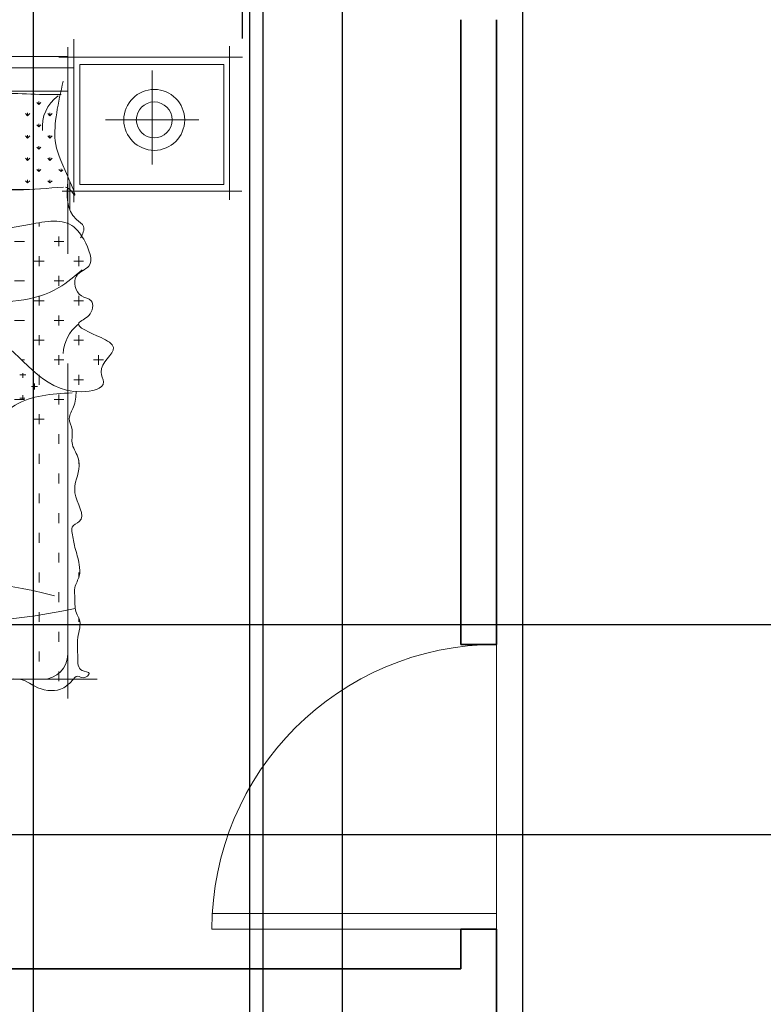
# Model space of a CAD drawing. Units: inches. Extents: x -438 to 102, y -60 to 1091.
# Tile 13 of 20: x -243 to -149, y 898 to 1022. Entities that reach past the tile are written whole.
import ezdxf

# ---------------------------------------------------------------- set-up
doc = ezdxf.new("R2010")
doc.units = ezdxf.units.IN
doc.header["$MEASUREMENT"] = 0
for name, color, linetype, lineweight, true_color in [('A-ANNO-DIMS', 217, 'Continuous', 18, 0x93278f), ('A-DOOR', 30, 'Continuous', 18, 0xf26722), ('A-WALL', 2, 'Continuous', 35, 0xf1eb1f)]:
    doc.layers.add(name, color=color, linetype=linetype, lineweight=lineweight, true_color=true_color)
doc.layers.add('Furniture', color=7, linetype='Continuous', lineweight=15)
doc.styles.get("Standard").update_dxf_attribs({"font": 'arial.ttf'})
doc.dimstyles.get("Standard").update_dxf_attribs({"dimtxt": 8, "dimasz": 0.18, "dimexe": 0.18, "dimexo": 0.0625, "dimgap": 0.09, "dimtad": 0, "dimtih": 1, "dimtoh": 1, "dimdec": 4, "dimzin": 0, "dimdsep": 46, "dimlunit": 3, "dimtxsty": 'Standard', "dimcen": 0.09, "dimadec": 0, "dimazin": 0, "dimtfac": 1, "dimtdec": 4, "dimtofl": 0, "dimtmove": 0, "dimatfit": 3, "dimfxl": 1, "dimtolj": 1, "dimtzin": 0, "dimarcsym": 0})

# ---------------------------------------------------------------- blocks, each defined once
blk = doc.blocks.new('BED-DOUBLE-WITH-NIGHTSTANDS')
for p, q in [((30.68, 0), (30.68, -20.6)), ((29.9, -1.01), (29.9, -27.13)), ((50.37, -20.33), (50.37, -0.9)), ((-30.74, -2.19), (29.9, -2.19)), ((51.99, -2.28), (28.76, -2.28)), ((30.68, -3.64), (-30.92, -3.64)), ((49.65, -3.21), (31.43, -3.21)), ((31.43, -3.21), (31.43, -18.39)), ((49.65, -18.39), (49.65, -3.21)), ((40.58, -3.96), (40.58, -15.85)), ((29.9, -6.59), (7.41, -6.59)), ((26.23, -8.26), (25.97, -8)), ((26.23, -8.27), (26.23, -7.89)), ((26.23, -8.26), (26.5, -8)), ((24.82, -9.68), (24.55, -9.41)), ((24.82, -9.68), (24.82, -9.3)), ((24.82, -9.68), (25.08, -9.41)), ((27.65, -9.68), (27.38, -9.41)), ((27.65, -9.68), (27.65, -9.3)), ((27.65, -9.68), (27.91, -9.41)), ((26.23, -11.09), (25.97, -10.83)), ((26.23, -11.09), (26.23, -10.72)), ((26.23, -11.09), (26.5, -10.83)), ((46.48, -10.21), (34.68, -10.21)), ((24.82, -12.51), (24.55, -12.24)), ((24.82, -12.51), (24.82, -12.13)), ((24.82, -12.51), (25.08, -12.24)), ((27.65, -12.51), (27.38, -12.24)), ((27.65, -12.51), (27.65, -12.13)), ((27.65, -12.51), (27.91, -12.24)), ((26.23, -13.92), (25.97, -13.66)), ((26.23, -13.92), (26.23, -13.55)), ((26.23, -13.92), (26.5, -13.66)), ((24.82, -15.34), (24.55, -15.07)), ((24.82, -15.34), (24.82, -14.96)), ((24.82, -15.34), (25.08, -15.07)), ((27.65, -15.34), (27.38, -15.07)), ((27.65, -15.34), (27.65, -14.96)), ((27.65, -15.34), (27.91, -15.07)), ((26.23, -16.75), (25.97, -16.48)), ((26.23, -16.75), (26.23, -16.38)), ((26.23, -16.75), (26.5, -16.48)), ((29.06, -16.75), (28.79, -16.48)), ((29.06, -16.75), (29.06, -16.38)), ((29.06, -16.75), (29.27, -16.54)), ((24.82, -18.16), (24.55, -17.9)), ((24.82, -18.16), (24.82, -17.79)), ((24.82, -18.16), (25.08, -17.9)), ((27.65, -18.16), (27.38, -17.9)), ((27.65, -18.16), (27.65, -17.79)), ((27.65, -18.16), (27.91, -17.9)), ((30.17, -21.62), (30.17, -17.94)), ((31.43, -18.39), (49.65, -18.39)), ((29.21, -19.21), (51.9, -19.21)), ((26.28, -23.69), (26.28, -23.21)), ((24.41, -25.57), (23.16, -25.57)), ((29.41, -25.57), (28.16, -25.57)), ((28.78, -26.19), (28.78, -24.94)), ((26.91, -28.07), (25.66, -28.07)), ((26.28, -28.69), (26.28, -27.44)), ((31.91, -28.07), (30.66, -28.07)), ((31.28, -28.69), (31.28, -27.44)), ((24.41, -30.57), (23.16, -30.57)), ((29.41, -30.57), (28.16, -30.57)), ((28.78, -31.19), (28.78, -29.94)), ((26.91, -33.07), (25.66, -33.07)), ((26.28, -33.69), (26.28, -32.44)), ((31.91, -33.07), (30.66, -33.07)), ((31.28, -33.69), (31.28, -32.44)), ((24.41, -35.57), (23.16, -35.57)), ((29.41, -35.57), (28.16, -35.57)), ((28.78, -36.19), (28.78, -34.94)), ((26.91, -38.07), (25.66, -38.07)), ((26.28, -38.69), (26.28, -37.44)), ((31.91, -38.07), (30.66, -38.07)), ((31.28, -38.69), (31.28, -37.44)), ((24.41, -40.57), (24.09, -40.57)), ((29.41, -40.57), (28.16, -40.57)), ((28.78, -41.19), (28.78, -39.94)), ((29.9, -41), (29.9, -83.36)), ((34.41, -40.57), (33.16, -40.57)), ((33.78, -41.19), (33.78, -39.94)), ((24.22, -42.82), (24.22, -42.22)), ((24.59, -42.45), (23.85, -42.45)), ((25.7, -44.29), (25.7, -43.56)), ((26.28, -43.69), (26.28, -42.44)), ((31.91, -43.07), (30.66, -43.07)), ((31.28, -43.69), (31.28, -42.44)), ((26.07, -43.92), (25.33, -43.92)), ((24.41, -45.57), (23.16, -45.57)), ((24.47, -45.4), (23.85, -45.4)), ((24.22, -45.56), (24.22, -45.03)), ((29.41, -45.57), (28.16, -45.57)), ((28.78, -46.19), (28.78, -44.94)), ((26.91, -48.07), (25.66, -48.07)), ((26.28, -48.69), (26.28, -47.44)), ((28.78, -51.19), (28.78, -49.94)), ((26.28, -53.69), (26.28, -52.44)), ((31.28, -53.69), (31.28, -53.25)), ((28.78, -56.19), (28.78, -54.94)), ((26.28, -58.69), (26.28, -57.44)), ((28.78, -61.19), (28.78, -59.94)), ((26.28, -63.69), (26.28, -62.44)), ((28.78, -66.19), (28.78, -64.94)), ((26.28, -68.69), (26.28, -67.44)), ((31.28, -68.1), (31.28, -67.44)), ((28.78, -71.19), (28.78, -69.94)), ((26.28, -73.69), (26.28, -72.44)), ((31.28, -73.69), (31.28, -73.16)), ((28.78, -76.19), (28.78, -74.94)), ((26.28, -78.69), (26.28, -77.44)), ((28.78, -81.19), (28.78, -79.94)), ((33.6, -80.93), (-28.29, -80.93))]:
    blk.add_line(p, q)
for radius in [3.85, 2.27]:
    blk.add_circle((40.84, -10.21), radius)
for centre, radius, start, end in [((31.35, -11.01), 4.66, 124.7345, 186.5526), ((24.21, 1.34), 20.36, 248.1857, 275.9106), ((34.27, -39.94), 4.94, 128.8354, 178.0038), ((14.99, -0.75), 72.97, 239.8126, 282.5472), ((9.5, -143.88), 75.85, 75.7143, 109.4459), ((26.75, -77.78), 3.15, 270, 0)]:
    blk.add_arc(centre, radius, start, end)
for points, knots in [([(29.35, -18.7), (25.48, -19.02), (19.22, -19.53), (10.28, -16.58), (3.99, -20.47), (0.06, -17.44), (0.95, -13.79), (1.87, -10.79), (0.46, -7.43), (6.72, -5.67), (11.66, -7.91), (18.15, -7.12), (22.47, -6.73), (26.14, -7.04), (28.33, -7.01), (29.06, -7.01)], [0, 0, 0, 0, 11.502554, 18.635017, 27.654655, 28.800011, 32.595859, 36.914018, 38.927328, 41.544104, 52.009639, 56.262652, 60.661637, 65.075538, 67.252844, 67.252844, 67.252844, 67.252844]), ([(29.32, -5.32), (28.7, -8.05), (27.69, -12.51), (29.2, -15.74), (31.39, -20.84), (30.11, -18.79), (29.6, -18.7)], [0, 0, 0, 0, 7.603099, 12.404488, 14.892294, 16.432626, 16.432626, 16.432626, 16.432626]), ([(29.9, -17.94), (29.78, -19.78), (29.64, -22.09), (32.27, -23.65), (31.79, -24.62), (31.53, -25.14)], [0, 0, 0, 0, 4.973031, 6.254082, 7.747585, 7.747585, 7.747585, 7.747585]), ([(31.93, -25.29), (32.57, -26.62), (33.59, -28.72), (30.29, -29.71), (31.01, -32.64), (33.35, -32.83), (32.92, -35.12), (30.08, -36.11), (33.79, -37.48), (36.78, -39.18), (33.39, -41.32), (35.07, -44.06), (26.87, -46.02), (20.99, -32.35), (2.1, -54.12), (-16.08, -50.43), (-31.16, -41.37), (-34.82, -50.79), (-35.75, -45.56), (-33.27, -44.57), (-36.07, -39.92), (-29.61, -39.91), (-31.05, -37.18), (-31.79, -35.41), (-31.67, -30.43), (-16.86, -30.76), (-35.73, -24.41), (-25.68, -23.88), (-16.82, -24.97), (2.34, -26.69), (17.46, -24.9), (30.09, -22.48), (31.54, -24.71), (31.93, -25.29)], [0, 0, 0, 0, 3.481099, 5.475811, 8.043407, 9.436812, 11.330727, 12.888379, 16.258255, 18.252967, 21.734596, 23.018392, 26.087149, 38.445812, 54.5649, 86.600283, 92.594507, 98.286547, 100.905288, 101.70342, 105.471876, 109.954916, 110.954151, 113.598333, 116.114301, 124.231953, 133.25029, 137.509046, 143.991555, 164.906349, 189.961005, 195.579007, 197.573325, 197.573325, 197.573325, 197.573325]), ([(31.74, -29.16), (30.78, -29.98), (26.99, -33.22), (21.81, -33.32), (17.94, -33.4)], [0, 0, 0, 0, 3.737027, 14.742384, 14.742384, 14.742384, 14.742384]), ([(30.47, -44.73), (27.88, -44.87), (22.83, -45.15), (16.72, -54.5), (5.64, -51.25), (-8.89, -48.66), (-19.85, -50.38), (-33.1, -52.54), (-34.5, -49.21), (-35, -48.01)], [0, 0, 0, 0, 7.385187, 14.402621, 29.694422, 35.583277, 59.348121, 65.733553, 69.320983, 69.320983, 69.320983, 69.320983]), ([(30.96, -44.51), (30.93, -45.19), (30.86, -46.38), (29.77, -47.93), (30.68, -49.44), (30.18, -51.19), (31.18, -52.55), (31.56, -54.75), (29.86, -57.22), (32.61, -60.74), (30.28, -61.5), (30.52, -62.88), (30.79, -64.38), (31.38, -66.15), (31.51, -67.95), (30.62, -69.27), (30.89, -70.9), (30.72, -72.32), (31.74, -73.74), (30.93, -75.81), (31.25, -77.78), (31.09, -79.97), (33.09, -80.01), (31.89, -81), (31.1, -80.32), (30.21, -81.43), (28.73, -82.66), (26.29, -82.31), (24.17, -80.73), (21.7, -80.78), (19.49, -82.4), (17.06, -81.88), (13.17, -82.17), (8.82, -81.36), (4.07, -80.77), (0.46, -83.09), (-2.79, -81.85), (-5.87, -81.65), (-14.3, -79.69), (-20.14, -80.18), (-31.55, -83.45), (-29.78, -79.6), (-32.81, -83.8), (-29.07, -82.96), (-24.85, -82.73), (-30.36, -81.5), (-32.31, -79.09), (-32.11, -72.2), (-27.72, -79.52), (-31.69, -72.6), (-28.72, -70.51), (-27.65, -65.93), (-35.2, -65.77), (-26.02, -64.12), (-35.79, -62.68), (-27.32, -61.35), (-31.95, -58.4), (-27.39, -55.21), (-31.95, -53.76), (-28.5, -51.75), (-29.55, -48.81), (-29.07, -42.18), (-29.13, -46.29), (-29.16, -48.01)], [0, 0, 0, 0, 2.033881, 3.581387, 5.07489, 6.704853, 8.655612, 9.757262, 13.24098, 16.903694, 18.063816, 18.788243, 20.635227, 22.875483, 24.324336, 25.871843, 27.320698, 29.140811, 29.950855, 32.312207, 34.847704, 36.565952, 37.541804, 38.447727, 39.194923, 40.100844, 41.912688, 45.194843, 46.251388, 49.875946, 51.496686, 54.215105, 56.7523, 63.316606, 67.484853, 70.581422, 75.324573, 76.965649, 79.915763, 100.671038, 102.483321, 104.317501, 106.523635, 109.038061, 111.571263, 115.809372, 117.667229, 122.411431, 125.445794, 129.976907, 132.758854, 136.424739, 139.918708, 143.481583, 147.135325, 151.002466, 153.252794, 157.23352, 159.244583, 161.905351, 164.097269, 169.015093, 172.531686, 172.531686, 172.531686, 172.531686])]:
    blk.add_open_spline(points, degree=3, knots=knots)
blk = doc.blocks.new('DOOR-SWING-36')
for p, q in [((-36, 0), (0, 0)), ((-2, 0), (-2, -36)), ((0, 0), (0, -36))]:
    blk.add_line(p, q)
blk.add_arc((0, 0), 36, 180, 270)
blk = doc.blocks.new('*D12')
at = {"layer": 'A-ANNO-DIMS', "color": 0, "lineweight": -2, "transparency": 16777216}
for p, q in [((-319.27, 1020.11), (-319.27, 1035.82)), ((-319.09, 1035.64), (-304.62, 1035.64)), ((-215.48, 1035.64), (-229.95, 1035.64)), ((-215.3, 1020.11), (-215.3, 1035.82))]:
    blk.add_line(p, q, dxfattribs=at)
at = {"layer": 'A-ANNO-DIMS', "color": 0, "transparency": 16777216}
for points in [[(-319.09, 1035.67), (-319.09, 1035.61), (-319.27, 1035.64)], [(-215.48, 1035.67), (-215.48, 1035.61), (-215.3, 1035.64)]]:
    blk.add_solid(points, dxfattribs=at)
at = {"layer": 'Defpoints', "color": 0, "transparency": 16777216}
for p in [(-215.3, 1035.64), (-319.27, 1020.04), (-215.3, 1020.04)]:
    blk.add_point(p, dxfattribs=at)
at = {"layer": 'A-ANNO-DIMS', "color": 0, "transparency": 16777216, "insert": (-267.28, 1035.64), "char_height": 8, "attachment_point": 5}
blk.add_mtext('\\A1;BED 8\'-8" TYP.', dxfattribs=at)
blk = doc.blocks.new('*D37')
at = {"layer": 'A-ANNO-DIMS', "color": 0, "lineweight": -2, "transparency": 16777216}
for p, q in [((-179.8, 234.94), (-179.8, 1079.58)), ((-134.08, 234.94), (-134.08, 1079.58)), ((-179.62, 1079.4), (-176.98, 1079.4)), ((-134.26, 1079.4), (-136.9, 1079.4))]:
    blk.add_line(p, q, dxfattribs=at)
at = {"layer": 'A-ANNO-DIMS', "color": 0, "transparency": 16777216}
for points in [[(-179.62, 1079.43), (-179.62, 1079.37), (-179.8, 1079.4)], [(-134.26, 1079.43), (-134.26, 1079.37), (-134.08, 1079.4)]]:
    blk.add_solid(points, dxfattribs=at)
at = {"layer": 'Defpoints', "color": 0, "transparency": 16777216}
for p in [(-134.08, 1079.4), (-179.8, 234.88), (-134.08, 234.88)]:
    blk.add_point(p, dxfattribs=at)
at = {"layer": 'A-ANNO-DIMS', "color": 0, "transparency": 16777216, "insert": (-156.94, 1079.4), "char_height": 8, "attachment_point": 5}
blk.add_mtext('\\A1;3\'-9 1/2"', dxfattribs=at)
blk = doc.blocks.new('*D44')
at = {"layer": 'A-ANNO-DIMS', "color": 0, "lineweight": -2, "transparency": 16777216}
for p, q in [((-64.71, 946), (-414.94, 946)), ((-414.76, 945.82), (-414.76, 936.94)), ((-414.76, 919.6), (-414.76, 928.48)), ((-64.71, 919.42), (-414.94, 919.42))]:
    blk.add_line(p, q, dxfattribs=at)
at = {"layer": 'A-ANNO-DIMS', "color": 0, "transparency": 16777216}
for points in [[(-414.79, 945.82), (-414.73, 945.82), (-414.76, 946)], [(-414.79, 919.6), (-414.73, 919.6), (-414.76, 919.42)]]:
    blk.add_solid(points, dxfattribs=at)
at = {"layer": 'Defpoints', "color": 0, "transparency": 16777216}
for p in [(-64.65, 946), (-414.76, 919.42), (-64.65, 919.42)]:
    blk.add_point(p, dxfattribs=at)
at = {"layer": 'A-ANNO-DIMS', "color": 0, "transparency": 16777216, "insert": (-414.76, 932.71), "char_height": 8, "attachment_point": 5}
blk.add_mtext('\\A1;2\'-2 1/2"', dxfattribs=at)
blk = doc.blocks.new('*D53')
at = {"layer": 'A-ANNO-DIMS', "color": 0, "lineweight": -2, "transparency": 16777216}
for p, q in [((-241.7, 824.44), (-241.7, 1079.58)), ((-214.37, 824.44), (-214.37, 1079.58)), ((-241.52, 1079.4), (-214.55, 1079.4)), ((-214.37, 1079.4), (-214.19, 1079.4))]:
    blk.add_line(p, q, dxfattribs=at)
at = {"layer": 'A-ANNO-DIMS', "color": 0, "transparency": 16777216}
for points in [[(-241.52, 1079.43), (-241.52, 1079.37), (-241.7, 1079.4)], [(-214.55, 1079.43), (-214.55, 1079.37), (-214.37, 1079.4)]]:
    blk.add_solid(points, dxfattribs=at)
at = {"layer": 'Defpoints', "color": 0, "transparency": 16777216}
for p in [(-214.37, 1079.4), (-241.7, 824.38), (-214.37, 824.38)]:
    blk.add_point(p, dxfattribs=at)
at = {"layer": 'A-ANNO-DIMS', "color": 0, "transparency": 16777216, "insert": (-194.08, 1079.4), "char_height": 8, "attachment_point": 5}
blk.add_mtext('\\A1;2\'-3 1/2"', dxfattribs=at)
blk = doc.blocks.new('*D61')
at = {"layer": 'A-ANNO-DIMS', "color": 0, "lineweight": -2, "transparency": 16777216}
for p, q in [((-212.65, 534.56), (-212.65, 1079.58)), ((-202.65, 534.56), (-202.65, 1079.58)), ((-212.65, 1079.4), (-212.83, 1079.4)), ((-202.83, 1079.4), (-212.47, 1079.4))]:
    blk.add_line(p, q, dxfattribs=at)
at = {"layer": 'A-ANNO-DIMS', "color": 0, "transparency": 16777216}
for points in [[(-212.47, 1079.43), (-212.47, 1079.37), (-212.65, 1079.4)], [(-202.83, 1079.43), (-202.83, 1079.37), (-202.65, 1079.4)]]:
    blk.add_solid(points, dxfattribs=at)
at = {"layer": 'Defpoints', "color": 0, "transparency": 16777216}
for p in [(-212.65, 1079.4), (-212.65, 534.5), (-202.65, 534.5)]:
    blk.add_point(p, dxfattribs=at)
at = {"layer": 'A-ANNO-DIMS', "color": 0, "transparency": 16777216, "insert": (-226.66, 1079.4), "char_height": 8, "attachment_point": 5}
blk.add_mtext('\\A1;0\'-10"', dxfattribs=at)

msp = doc.modelspace()

# ---------------------------------------------------------------- linework, layer by layer
at = {"layer": 'A-WALL'}
for p, q in [((-187.64649, 1022.49939), (-187.64649, 943.50091)), ((-183.14649, 1022.49939), (-183.14649, 943.50091)), ((-183.14649, 943.50091), (-187.64649, 943.50091)), ((-183.14649, 907.50091), (-187.64649, 907.50091)), ((-187.64649, 907.50091), (-187.64649, 902.49939)), ((-183.14649, 907.50091), (-183.14649, 893.74862)), ((-187.64649, 902.49939), (-310.7047, 902.49939))]:
    msp.add_line(p, q, dxfattribs=at)

# ---------------------------------------------------------------- block references
at = {"layer": 'A-DOOR', "rotation": 270.0000000000001}
msp.add_blockref('DOOR-SWING-36', (-183.14649, 907.50091), dxfattribs=at)
at = {"layer": 'Furniture'}
msp.add_blockref('BED-DOUBLE-WITH-NIGHTSTANDS', (-267.285, 1020.04), dxfattribs=at)

# ---------------------------------------------------------------- dimensions: what is measured, and where the dimension line sits
at = {"layer": 'A-ANNO-DIMS'}
for base, p1, p2, picture, middle in [((-214.3672, 1079.39939), (-241.69558, 824.37939), (-214.3672, 824.37939), '*D53', (-194.07537, 1079.39939)), ((-134.07948, 1079.39939), (-179.79585, 234.87846), (-134.07948, 234.87846), '*D37', (-156.93767, 1079.39939)), ((-212.64649, 1079.39939), (-202.64649, 534.49939), (-212.64649, 534.49939), '*D61', (-226.65728, 1079.39939))]:
    dim = msp.add_linear_dim(base=base, p1=p1, p2=p2, dimstyle='Standard', override={"dimdec": 1, "dimlfac": 1, "dimrnd": 0, "dimzin": 1, "dimdsep": 46, "dimlunit": 4, "dimfrac": 2}, dxfattribs=at)
    dim.commit()
    dim.dimension.update_dxf_attribs({"geometry": picture, "text_midpoint": middle})
dim = msp.add_linear_dim(base=(-215.29994, 1035.63825), p1=(-319.26918, 1020.04286), p2=(-215.29994, 1020.04286), text='BED <> TYP.', dimstyle='Standard', override={"dimdec": 1, "dimlfac": 1, "dimrnd": 0, "dimzin": 1, "dimdsep": 46, "dimlunit": 4, "dimfrac": 2}, dxfattribs=at)
dim.commit()
dim.dimension.update_dxf_attribs({"geometry": '*D12', "text_midpoint": (-267.28456, 1035.63825)})
dim = msp.add_linear_dim(base=(-414.76009, 919.41905), p1=(-64.64649, 945.99939), p2=(-64.64649, 919.41905), angle=90, dimstyle='Standard', override={"dimdec": 1, "dimlfac": 1, "dimrnd": 0, "dimzin": 1, "dimdsep": 46, "dimlunit": 4, "dimfrac": 2}, dxfattribs=at)
dim.commit()
dim.dimension.update_dxf_attribs({"geometry": '*D44', "text_midpoint": (-414.76009, 932.70922)})

doc.saveas('drawing.dxf')
